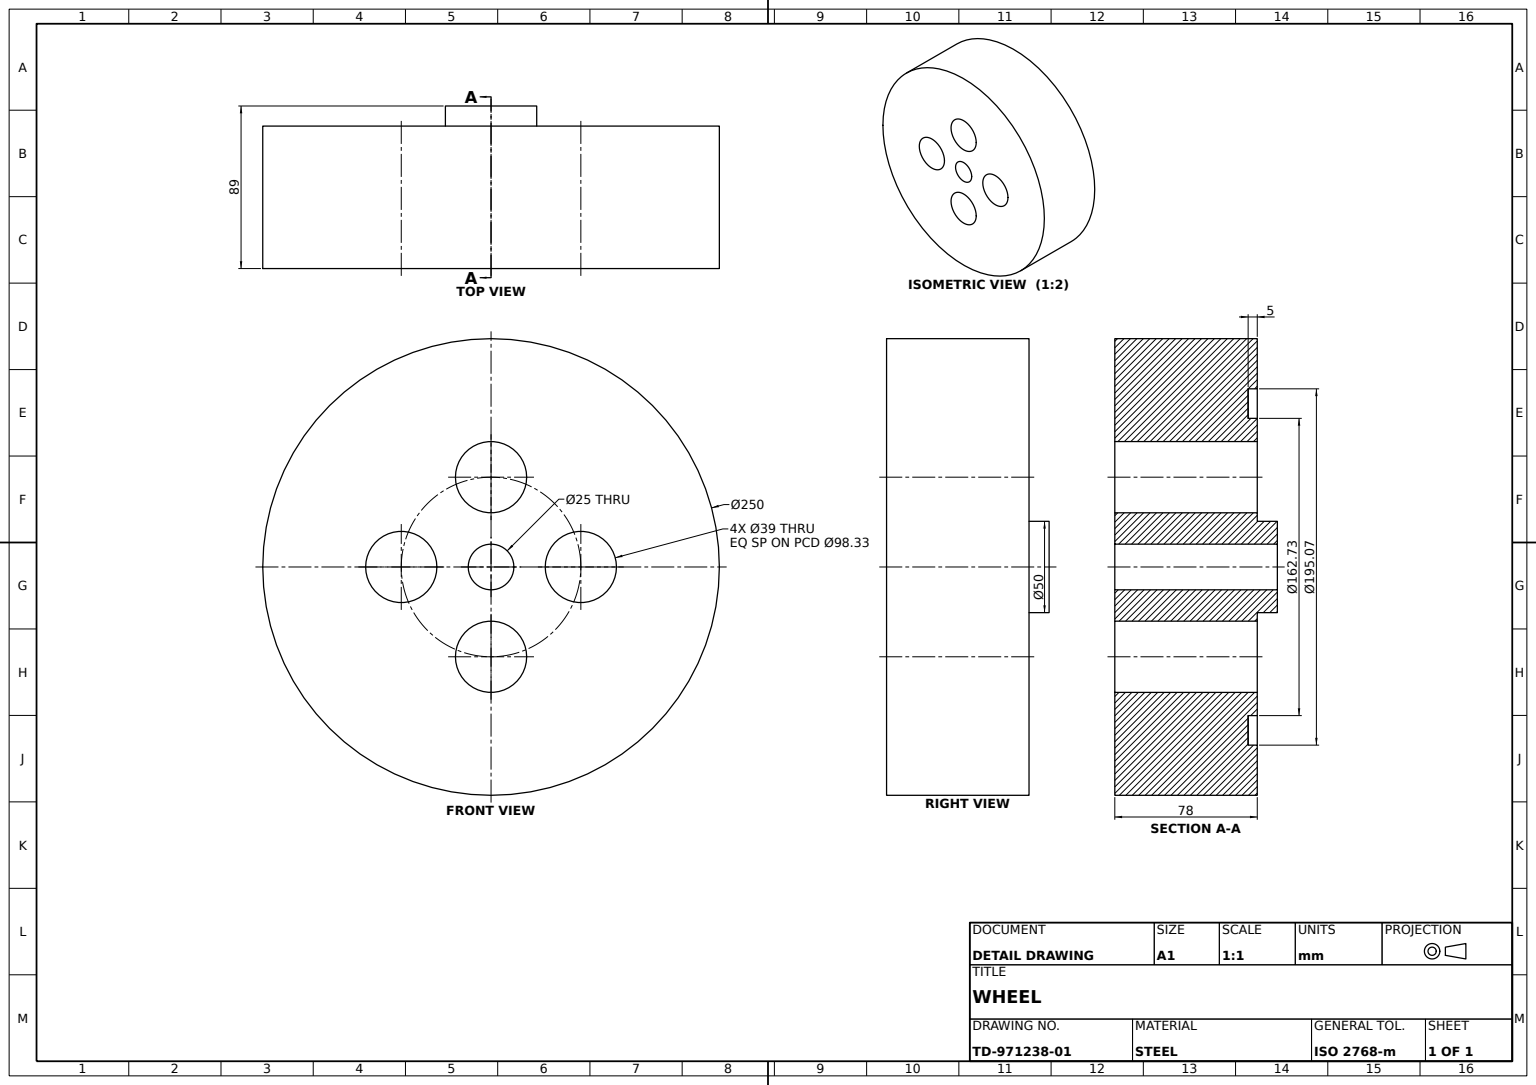
from build123d import *

# Parameters (mm, degrees)
WHEEL_DISC_SKETCH_R        = 125
WHEEL_DISC_250_DEPTH       = 78
FACE_RECESS_SKETCH_R       = 97.533404225
FACE_RECESS_SKETCH_R_2     = 81.367148925
FACE_RECESS_5MM_DEPTH      = 5
LIGHTENING_HOLE_1_SKETCH_R = 19.5
LIGHTENING_HOLE_1_39_DEPTH = 78
LIGHTENING_HOLE_2_SKETCH_R = 19.5
LIGHTENING_HOLE_2_39_DEPTH = 78
LIGHTENING_HOLE_3_SKETCH_R = 19.5
LIGHTENING_HOLE_3_39_DEPTH = 78
LIGHTENING_HOLE_4_SKETCH_R = 19.5
LIGHTENING_HOLE_4_39_DEPTH = 78
HUB_BOSS_SKETCH_R          = 25
HUB_BOSS_SKETCH_R_2        = 12.5
HUB_BOSS_50_DEPTH          = 16
CENTRE_START               = -78
CENTRE_CUT_SKETCH_R        = 12.5
CENTRE_CUT_DEPTH           = 78


with BuildPart() as part:
    # Wheel Disc Sketch → Wheel Disc Ø250 (new body)
    with BuildSketch(Plane.XY):
        Circle(WHEEL_DISC_SKETCH_R)
    extrude(amount=-WHEEL_DISC_250_DEPTH)

    # Face Recess Sketch → Face Recess 5mm (cut)
    with BuildSketch(Plane.XY):
        Circle(FACE_RECESS_SKETCH_R)
        Circle(FACE_RECESS_SKETCH_R_2, mode=Mode.SUBTRACT)
    extrude(amount=-FACE_RECESS_5MM_DEPTH, mode=Mode.SUBTRACT)

    # Lightening Hole 1 Sketch → Lightening Hole 1 Ø39 (cut)
    with BuildSketch(Plane.XY):
        with Locations((0, 49.162629863)):
            Circle(LIGHTENING_HOLE_1_SKETCH_R)
    extrude(amount=-LIGHTENING_HOLE_1_39_DEPTH, mode=Mode.SUBTRACT)

    # Lightening Hole 2 Sketch → Lightening Hole 2 Ø39 (cut)
    with BuildSketch(Plane.XY):
        with Locations((49.162629863, 0)):
            Circle(LIGHTENING_HOLE_2_SKETCH_R)
    extrude(amount=-LIGHTENING_HOLE_2_39_DEPTH, mode=Mode.SUBTRACT)

    # Lightening Hole 3 Sketch → Lightening Hole 3 Ø39 (cut)
    with BuildSketch(Plane.XY):
        with Locations((0, -49.162629863)):
            Circle(LIGHTENING_HOLE_3_SKETCH_R)
    extrude(amount=-LIGHTENING_HOLE_3_39_DEPTH, mode=Mode.SUBTRACT)

    # Lightening Hole 4 Sketch → Lightening Hole 4 Ø39 (cut)
    with BuildSketch(Plane.XY):
        with Locations((-49.162629863, 0)):
            Circle(LIGHTENING_HOLE_4_SKETCH_R)
    extrude(amount=-LIGHTENING_HOLE_4_39_DEPTH, mode=Mode.SUBTRACT)

    # Hub Boss Sketch → Hub Boss Ø50 (add)
    with BuildSketch(Plane.XY.offset(-5)):
        Circle(HUB_BOSS_SKETCH_R)
        Circle(HUB_BOSS_SKETCH_R_2, mode=Mode.SUBTRACT)
    extrude(amount=HUB_BOSS_50_DEPTH)

    # Centre Cut Sketch → Centre Cut (cut)
    with BuildSketch(Plane.XY.offset(CENTRE_START)):
        Circle(CENTRE_CUT_SKETCH_R)
    extrude(amount=CENTRE_CUT_DEPTH, mode=Mode.SUBTRACT)


solid = part.part
